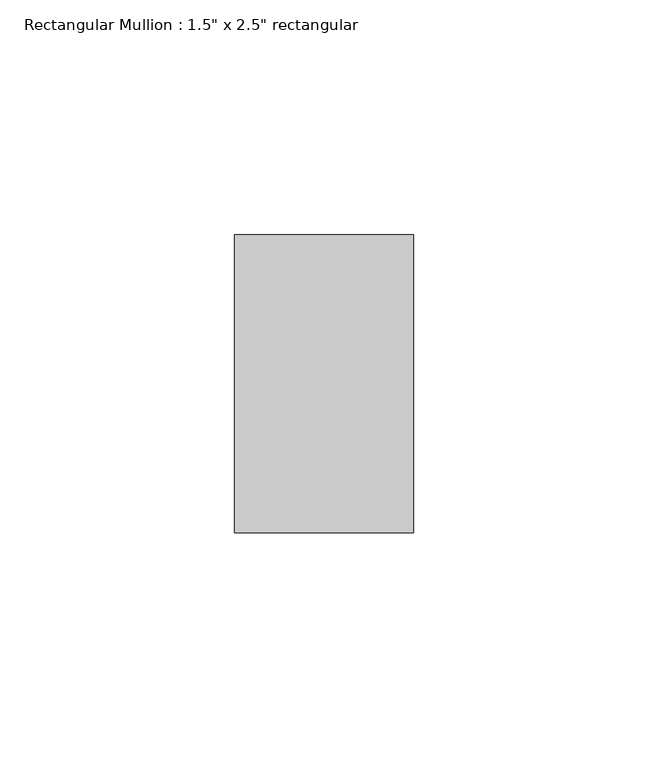
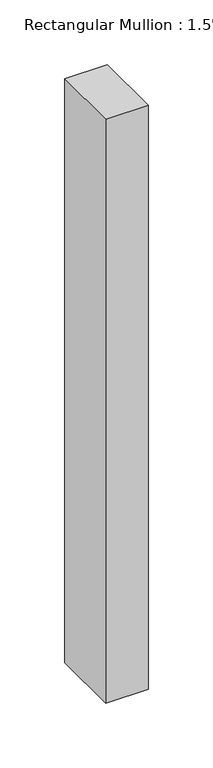
"""IFC4 building model written with IfcOpenShell, lengths in millimetres: member geometry."""

from ifc_helpers import new_model, si_unit, frame, origin, place, context, project, spatial, polyline, outline, extrude, source, transform, mapped, element, save


def member_6a7c88b6(model_context):
    return source(origin(), model_context, "Body", "SweptSolid", [
        extrude(outline(polyline([(19.05, 31.75), (19.05, -31.75), (-19.05, -31.75), (-19.05, 31.75), (19.05, 31.75)])), frame((0.0, 0.0, -552.4500003), z_axis=(0.0, 0.0, 1.0), x_axis=(1.0, 0.0, 0.0)), (0.0, 0.0, 1.0), 552.4500003),
    ])


if __name__ == "__main__":
    model = new_model("IFC4")
    model_context = context("Model", 3, world=origin())
    ifc_project = project(units=[si_unit("LENGTHUNIT", "METRE", prefix="MILLI")], contexts=[model_context])
    site = spatial("IfcSite", under=ifc_project)
    building = spatial("IfcBuilding", under=site)
    placement = place(None, origin())
    member_shape = member_6a7c88b6(model_context)
    element("IfcMember", 1, ObjectType="Rectangular Mullion : 1.5\" x 2.5\" rectangular", at=placement, inside=building, context=model_context, shape_type="MappedRepresentation", body=[
        mapped(member_shape, transform((0.0, 0.0, 0.0), x_axis=(1.0, 0.0, 0.0), y_axis=(0.0, 1.0, 0.0), z_axis=(0.0, 0.0, 1.0))),
    ])
    save(model, "model.ifc")

# Revit data of these elements
# Type "Rectangular Mullion : 1.5\" x 2.5\" rectangular"
#   built-in parameter 1007304 = 0.208333 (stored number, unit not read)
#   built-in parameter 1007301 = 0.0625 (stored number, unit not read)
#   built-in parameter 1007300 = 0.0625 (stored number, unit not read)
# Element 1 (IfcMember, "Rectangular Mullion : 1.5\" x 2.5\" rectangular")
#   Materials on its faces: "Aluminum"
# Materials
#   "Aluminum": class "Metal", colour RGB 247 247 247, transparency 0, Description = "Aluminum 6061", Cost = 0
